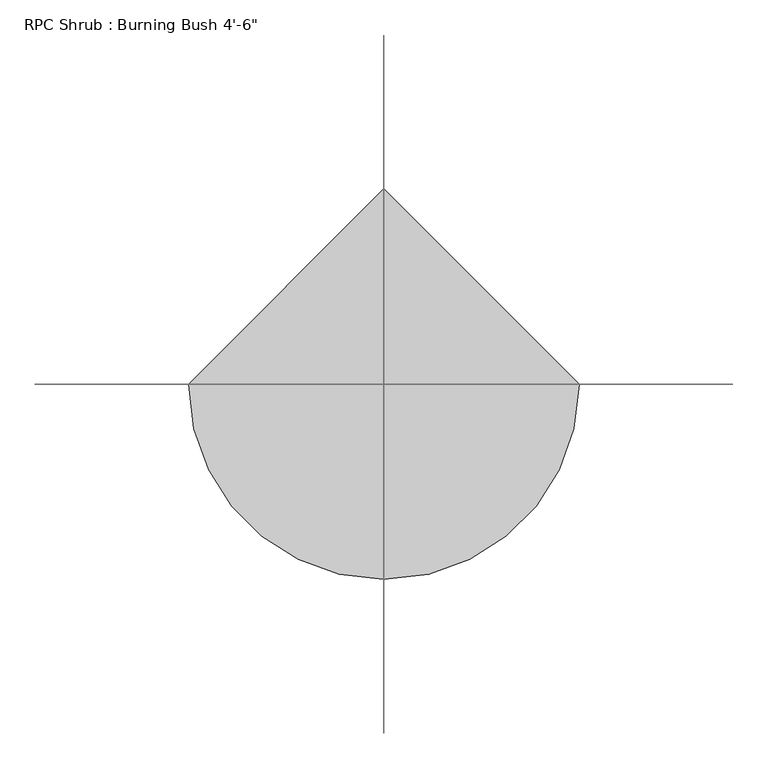
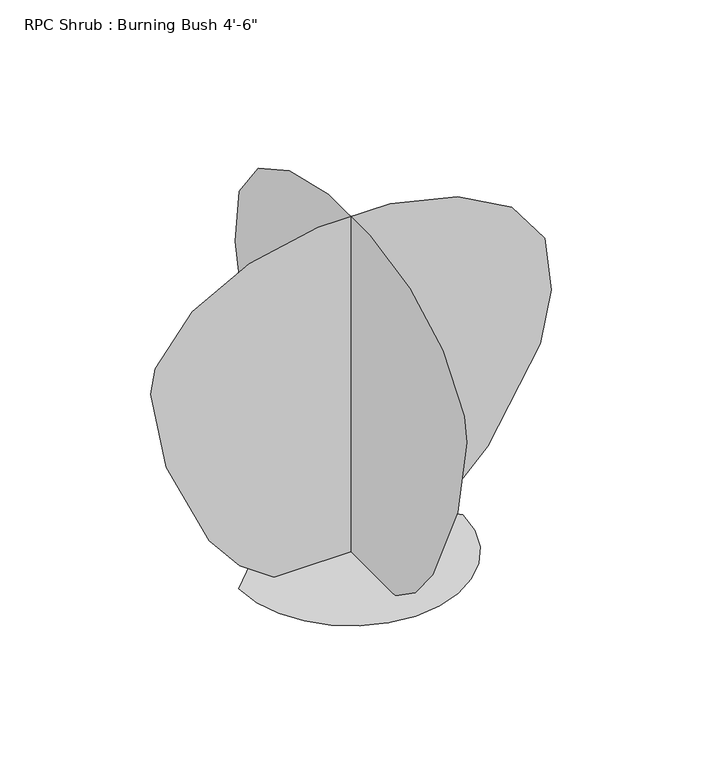
"""IFC4 building model written with IfcOpenShell, lengths in millimetres: geographic element geometry."""

from ifc_helpers import new_model, si_unit, origin, place, context, project, spatial, triangles, source, transform, mapped, element, save


def geographic_element_ca6e1e19(model_context):
    return source(origin(), model_context, "Body", "Tessellation", [
        triangles([(-433.0060553, 0.0, 9.6e-06), (-421.5583165, -99.2161097, 9.6e-06), (-388.9574358, -190.3303883, 9.6e-06), (-337.809504, -270.7307133, 9.6e-06), (-270.7307133, -337.809504, 9.6e-06), (-190.3301339, -388.9574358, 9.6e-06), (-99.2161097, -421.5583165, 9.6e-06), (1.89e-05, -433.0060553, 9.6e-06), (99.2161097, -421.5583165, 9.6e-06), (190.3303883, -388.9574358, 9.6e-06), (270.7307133, -337.809504, 9.6e-06), (337.8120475, -270.7307133, 9.6e-06), (388.9574358, -190.3301339, 9.6e-06), (421.5583165, -99.2161097, 9.6e-06), (433.0060553, 3.79e-05, 9.6e-06), (-5.68e-05, 433.0060553, 9.6e-06), (0.0014009, -430.765785, 94.2524501), (0.0014009, -546.9046263, 237.6063543), (0.0014009, -714.237145, 595.0121913), (0.0014009, -774.5366621, 915.4404888), (0.0014009, -756.8862133, 1012.5699526), (0.0014009, -613.7091242, 1195.6605938), (0.0014009, -392.9985772, 1314.6594349), (0.0014009, -126.9008115, 1371.5986919), (0.0014009, 152.4422576, 1368.5125431), (0.0014009, 412.8816659, 1307.4357479), (0.0014009, 622.2765518, 1190.4028479), (0.0014009, 748.478805, 1019.4483118), (0.0014009, 774.5341187, 800.0204264), (0.0014009, 730.9985493, 593.4373964), (0.0014009, 528.3042355, 247.0045997), (0.0014009, 284.5635354, 0.0), (0.0014009, -297.0654067, 0.7142016), (-430.7632416, -0.0013164, 94.2524501), (-546.9020828, -0.001325, 237.6063543), (-714.2346016, -0.0013463, 595.0121913), (-774.5341187, -0.0013654, 915.4404888), (-756.8836699, -0.0013711, 1012.5699526), (-613.7065807, -0.0013821, 1195.6605938), (-392.9960338, -0.0013892, 1314.6594349), (-126.8977685, -0.0013925, 1371.5986919), (152.4450554, -0.0013924, 1368.5125431), (412.8867528, -0.0013887, 1307.4357479), (622.2790226, -0.0013817, 1190.4028479), (748.4813484, -0.0013716, 1019.4483118), (774.5366621, -0.0013585, 800.0204264), (731.0010927, -0.0013462, 593.4373964), (528.3067789, -0.0013255, 247.0045997), (284.5660788, -0.0013108, 6.01e-05), (-297.0628633, -0.0013108, 0.7142625)], [[15, 16, 1], [14, 15, 1], [14, 1, 2], [13, 14, 2], [13, 2, 3], [13, 3, 4], [12, 13, 4], [11, 12, 4], [11, 4, 5], [11, 5, 6], [11, 6, 7], [11, 7, 8], [11, 8, 9], [11, 9, 10], [32, 33, 17], [32, 17, 18], [31, 32, 18], [31, 18, 19], [30, 31, 19], [29, 30, 19], [28, 29, 19], [27, 28, 19], [26, 27, 19], [25, 26, 19], [24, 25, 19], [23, 24, 19], [22, 23, 19], [21, 22, 19], [21, 19, 20], [49, 50, 34], [49, 34, 35], [48, 49, 35], [48, 35, 36], [47, 48, 36], [46, 47, 36], [45, 46, 36], [44, 45, 36], [43, 44, 36], [42, 43, 36], [41, 42, 36], [40, 41, 36], [39, 40, 36], [38, 39, 36], [38, 36, 37]], closed=False),
    ])


if __name__ == "__main__":
    model = new_model("IFC4")
    model_context = context("Model", 3, world=origin())
    ifc_project = project(units=[si_unit("LENGTHUNIT", "METRE", prefix="MILLI")], contexts=[model_context])
    site = spatial("IfcSite", under=ifc_project)
    building = spatial("IfcBuilding", under=site)
    placement = place(None, origin())
    geographic_element_shape = geographic_element_ca6e1e19(model_context)
    element("IfcGeographicElement", 1, ObjectType="RPC Shrub : Burning Bush 4'-6\"", at=placement, inside=building, context=model_context, shape_type="MappedRepresentation", body=[
        mapped(geographic_element_shape, transform((0.0, 0.0, 0.0), x_axis=(1.0, 0.0, 0.0), y_axis=(0.0, 1.0, 0.0), z_axis=(0.0, 0.0, 1.0))),
    ])
    save(model, "model.ifc")

# Revit data of these elements
# Type "RPC Shrub : Burning Bush 4'-6\""
#   Type Comments = "Burning Bush"
#   built-in parameter 1005198 = "{2, 15},{39, RPC-16-FVGW-0UXX-7JA7-N000-ST1L-LVER-AU},{1, 0},{1, 0},{2, 13},{1, 8},{5, Color},{1, 0},{1, 0},{3, 0.8},{3, 0.8},{3, 0.8},{1, 8},{7, BBoxMin},{1, 0},{1, 0},{1, 0},{1, 0},{1, 0},{1, 8},{7, BBoxMax},{1, 0},{1, 0},{1, 0},{1, 0},{1, 0},{2, 11},{9, RPCTypeId},{1, 0},{1, 0},{39, RPC-16-FVGW-0UXX-7JA7-N000-ST1L-LVER-AU},{1, 6},{14, RPCPlantHeight},{1, 0},{1, 0},{3, 4.5},{2, 11},{7, keyword},{1, 0},{1, 0},{35, :RPCs:Shrubs & Grasses:Geometry:RPC},{2, 11},{8, category},{1, 0},{1, 0},{16, Shrubs & Grasses},{2, 11},{12, LocalizedUID},{1, 0},{1, 0},{12, Burning Bush},{2, 14},{6, Height},{1, 0},{1, 0},{3, 4.5},{1, 2},{16, Cast Reflections},{1, 0},{1, 0},{1, 0},{1, 2},{12, Cast Shadows},{1, 0},{1, 0},{1, 1},{1, 2},{9, Lock View},{1, 0},{1, 0},{1, 0},{1, 4},{5, ViewC},{1, 0},{1, 0},{1, 0},{21, assetlibrary_base.fbx},{1, 5},"
#   built-in parameter 1005195 = "RPC-16-FVGW-0UXX-7JA7-N000-ST1L-LVER-AU"
#   Assembly Code = "G2050500"
#   Height = 4' - 6"
#   Default Elevation = 0
